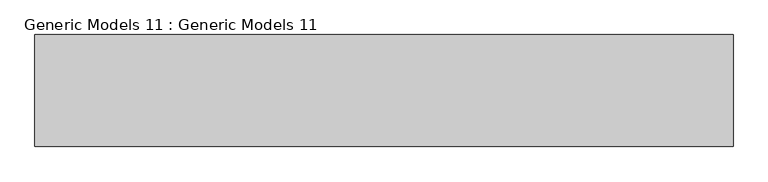
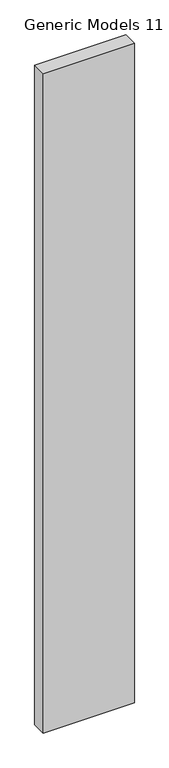
"""IFC4 building model written with IfcOpenShell, lengths in millimetres: proxy geometry, Generic Models 11 : Generic Models 11."""

from ifc_helpers import new_model, si_unit, frame, origin, place, context, project, spatial, polyline, outline, extrude, source, transform, mapped, element, save


def generic_models_11_generic_models_11_1ba3c33d(model_context):
    return source(origin(), model_context, "Body", "SweptSolid", [
        extrude(outline(polyline([(-3407.5048402, -3907.1858351), (-3407.5048402, -4516.7858351), (-7217.603092, -4516.7858351), (-7217.603092, -3907.1858351), (-3407.5048402, -3907.1858351)])), frame((0.0, 0.0, 3372.1768448), z_axis=(0.0, 0.0, 1.0), x_axis=(1.0, 0.0, 0.0)), (0.0, 0.0, 1.0), 29116.3557887),
    ])


if __name__ == "__main__":
    model = new_model("IFC4")
    model_context = context("Model", 3, world=origin())
    ifc_project = project(units=[si_unit("LENGTHUNIT", "METRE", prefix="MILLI")], contexts=[model_context])
    site = spatial("IfcSite", under=ifc_project)
    building = spatial("IfcBuilding", under=site)
    placement = place(None, origin())
    generic_models_11_generic_models_11_shape = generic_models_11_generic_models_11_1ba3c33d(model_context)
    element("IfcBuildingElementProxy", 1, Name="Generic Models 11 : Generic Models 11", ObjectType="Generic Models 11 : Generic Models 11", at=placement, inside=building, context=model_context, shape_type="MappedRepresentation", body=[
        mapped(generic_models_11_generic_models_11_shape, transform((0.0, 0.0, 0.0), x_axis=(1.0, 0.0, 0.0), y_axis=(0.0, 1.0, 0.0), z_axis=(0.0, 0.0, 1.0))),
    ])
    save(model, "model.ifc")
